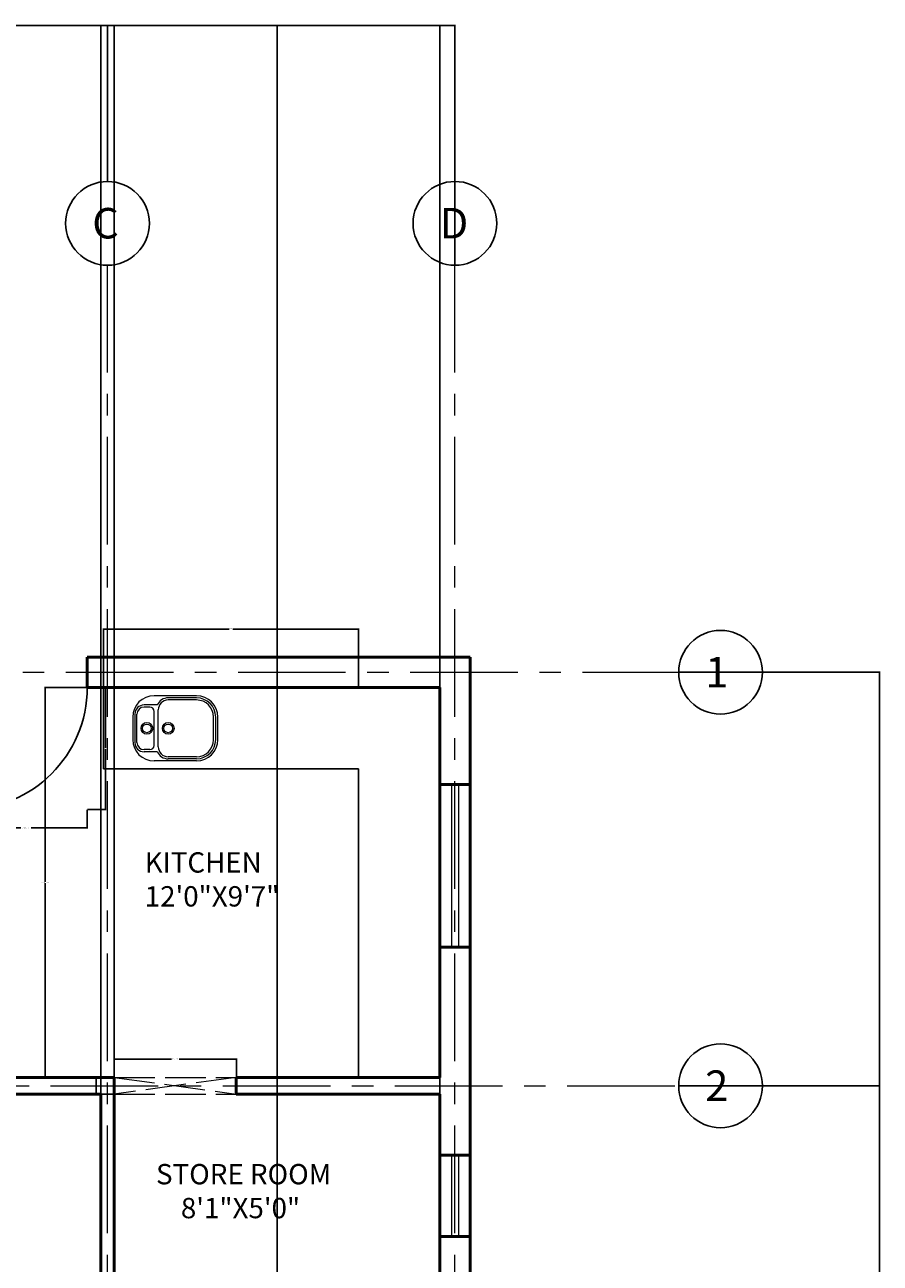
# Model space of a CAD drawing. Units: inches. Extents: x 10696 to 11614, y 5787 to 6498.
# Tile 9 of 9: x 11361 to 11614, y 6132 to 6498. Entities that reach past the tile are written whole.
import ezdxf

# ---------------------------------------------------------------- set-up
doc = ezdxf.new("R2010")
doc.units = ezdxf.units.IN
doc.linetypes.add('ACAD_ISO02W100', pattern=[15, 12, -3])
doc.linetypes.add('CENTER', pattern=[50.8, 31.75, -6.35, 6.35, -6.35])
for name, color, linetype, lineweight in [('A-ANNO-DIMS', 2, 'Continuous', 18), ('A-AREA-IDEN', 7, 'Continuous', 25), ('A-DOOR', 3, 'Continuous', 25), ('A-FLOR-CASE', 32, 'Continuous', 25), ('A-FLOR-FIXT', 9, 'Continuous', 20), ('A-GLAZ', 4, 'Continuous', 20), ('A-GRID', 1, 'CENTER', 18), ('A-GRID-IDEN', 1, 'Continuous', 25), ('A-WALL', 7, 'Continuous', 50), ('A-WALL-OVHD', 7, 'ACAD_ISO02W100', 18)]:
    doc.layers.add(name, color=color, linetype=linetype, lineweight=lineweight)
doc.styles.get("Standard").update_dxf_attribs({"font": 'arial.ttf'})
doc.dimstyles.get("Standard").update_dxf_attribs({"dimtxt": 0.18, "dimasz": 0.18, "dimexe": 0.18, "dimexo": 0.0625, "dimgap": 0.09, "dimtad": 0, "dimtih": 1, "dimtoh": 1, "dimdec": 4, "dimzin": 0, "dimdsep": 46, "dimtxsty": 'Standard', "dimcen": 0.09, "dimadec": 0, "dimazin": 0, "dimtfac": 1, "dimtdec": 4, "dimtofl": 0, "dimtmove": 0, "dimatfit": 3, "dimfxl": 1, "dimtolj": 1, "dimtzin": 0, "dimarcsym": 0})

# ---------------------------------------------------------------- blocks, each defined once
blk = doc.blocks.new('A$C29210457')
for p, q in [((0.63, 0.644), (0.21, 0.644)), ((0.63, 0.623), (0.35, 0.623)), ((0.242, 0.553), (0.112, 0.553)), ((0.168, 0.532), (0.112, 0.532)), ((0.14, 0.532), (0.14, 0.532)), ((0.21, 0.154), (0.21, 0.49)), ((0.252, 0.14), (0.252, 0.504)), ((0.63, 0.602), (0.35, 0.602)), ((0, 0.434), (0, 0.21)), ((0.021, 0.462), (0.021, 0.182)), ((0.042, 0.182), (0.042, 0.462)), ((0.798, 0.21), (0.798, 0.434)), ((0.819, 0.21), (0.819, 0.434)), ((0.84, 0.21), (0.84, 0.434)), ((0.168, 0.112), (0.112, 0.112)), ((0.242, 0.091), (0.112, 0.091)), ((0.14, 0.112), (0.14, 0.112)), ((0.63, 0), (0.21, 0)), ((0.63, 0.042), (0.35, 0.042)), ((0.63, 0.021), (0.35, 0.021))]:
    blk.add_line(p, q)
for centre, radius in [((0.14, 0.322), 0.0574), ((0.35, 0.322), 0.0574), ((0.14, 0.322), 0.0427), ((0.35, 0.322), 0.0427)]:
    blk.add_circle(centre, radius)
for centre, radius, start, end in [((0.21, 0.434), 0.21, 90, 180), ((0.35, 0.504), 0.119, 90.0649, 155.684), ((0.63, 0.434), 0.21, 0, 90), ((0.63, 0.434), 0.189, 0, 90), ((0.112, 0.462), 0.091, 90.0958, 180), ((0.112, 0.462), 0.07, 90, 180), ((0.168, 0.49), 0.042, 0, 90), ((0.35, 0.504), 0.098, 90, 180), ((0.63, 0.434), 0.168, 0, 90), ((0.21, 0.21), 0.21, 180, 270), ((0.112, 0.182), 0.091, 180, 270), ((0.112, 0.182), 0.07, 180, 270), ((0.168, 0.154), 0.042, 270, 0), ((0.35, 0.14), 0.098, 180, 270), ((0.63, 0.21), 0.21, 270, 0), ((0.63, 0.21), 0.168, 270, 0), ((0.63, 0.21), 0.189, 270, 0), ((0.35, 0.14), 0.119, 204.316, 269.978)]:
    blk.add_arc(centre, radius, start, end)
blk = doc.blocks.new('A$C292E2DA8')
at = {"xscale": 729, "yscale": 729, "zscale": 729}
blk.add_blockref('A$C29210457', (0, 0), dxfattribs=at)
blk = doc.blocks.new('DOOR-SINGLE-36-KITCHEN')
blk.add_line((0, 36), (0, 0))
blk.add_arc((0, 36), 36, 270, 0)
blk = doc.blocks.new('WIN-GLAZ-24')
for p, q in [((0, 24), (0, 0)), ((2, 24), (2, 0))]:
    blk.add_line(p, q)
blk = doc.blocks.new('WIN-GLAZ-48')
for p, q in [((0, 48), (0, 0)), ((2, 48), (2, 0))]:
    blk.add_line(p, q)
blk = doc.blocks.new('KITCHEN-COUNTER-L')
for p, q in [((0, 91), (0, 115)), ((0, 91), (75.19, 91)), ((75.19, 0), (75.19, 91))]:
    blk.add_line(p, q)
blk = doc.blocks.new('OPENING-OVHD-36X5')
for p, q in [((0, 5), (36, 5)), ((36, 5), (0, 0)), ((0, 5), (36, 0)), ((0, 0), (36, 0))]:
    blk.add_line(p, q)
blk = doc.blocks.new('*D48')
at = {"layer": 'A-ANNO-DIMS', "color": 0, "lineweight": -2, "transparency": 16777216}
for p, q in [((11343.77, 6266.01), (11343.77, 6260.49)), ((11379.77, 6266.01), (11379.77, 6260.49)), ((11343.95, 6260.67), (11360.24, 6260.67)), ((11379.59, 6260.67), (11363.29, 6260.67))]:
    blk.add_line(p, q, dxfattribs=at)
at = {"layer": 'A-ANNO-DIMS', "color": 0, "transparency": 16777216}
for points in [[(11343.95, 6260.7), (11343.95, 6260.64), (11343.77, 6260.67)], [(11379.59, 6260.7), (11379.59, 6260.64), (11379.77, 6260.67)]]:
    blk.add_solid(points, dxfattribs=at)
at = {"layer": 'Defpoints', "color": 0, "transparency": 16777216}
for p in [(11343.77, 6266.07), (11379.77, 6266.07), (11379.77, 6260.67)]:
    blk.add_point(p, dxfattribs=at)
at = {"layer": 'A-ANNO-DIMS', "color": 0, "transparency": 16777216, "insert": (11361.77, 6260.67), "char_height": 0.18, "attachment_point": 5}
blk.add_mtext('\\A1;KITCHEN DOOR 36 TYP.', dxfattribs=at)
blk = doc.blocks.new('*D49')
at = {"layer": 'A-ANNO-DIMS', "color": 0, "lineweight": -2, "transparency": 16777216}
for p, q in [((11379.83, 6302.07), (11385.35, 6302.07)), ((11385.17, 6301.89), (11385.17, 6284.25)), ((11385.17, 6266.25), (11385.17, 6283.89)), ((11379.83, 6266.07), (11385.35, 6266.07))]:
    blk.add_line(p, q, dxfattribs=at)
at = {"layer": 'A-ANNO-DIMS', "color": 0, "transparency": 16777216}
for points in [[(11385.14, 6301.89), (11385.2, 6301.89), (11385.17, 6302.07)], [(11385.14, 6266.25), (11385.2, 6266.25), (11385.17, 6266.07)]]:
    blk.add_solid(points, dxfattribs=at)
at = {"layer": 'Defpoints', "color": 0, "transparency": 16777216}
for p in [(11379.77, 6302.07), (11385.17, 6302.07), (11379.77, 6266.07)]:
    blk.add_point(p, dxfattribs=at)
at = {"layer": 'A-ANNO-DIMS', "color": 0, "transparency": 16777216, "insert": (11385.17, 6284.07), "char_height": 0.18, "attachment_point": 5}
blk.add_mtext('\\A1;36 TYP.', dxfattribs=at)
blk = doc.blocks.new('*D58')
at = {"layer": 'A-ANNO-DIMS', "color": 0, "lineweight": -2, "transparency": 16777216}
for p, q in [((11384.52, 6302.07), (11367.15, 6302.07)), ((11367.33, 6301.89), (11367.33, 6244.75)), ((11367.33, 6187.25), (11367.33, 6244.39)), ((11384.52, 6187.07), (11367.15, 6187.07))]:
    blk.add_line(p, q, dxfattribs=at)
at = {"layer": 'A-ANNO-DIMS', "color": 0, "transparency": 16777216}
for points in [[(11367.3, 6301.89), (11367.36, 6301.89), (11367.33, 6302.07)], [(11367.3, 6187.25), (11367.36, 6187.25), (11367.33, 6187.07)]]:
    blk.add_solid(points, dxfattribs=at)
at = {"layer": 'Defpoints', "color": 0, "transparency": 16777216}
for p in [(11367.33, 6302.07), (11384.58, 6302.07), (11384.58, 6187.07)]:
    blk.add_point(p, dxfattribs=at)
at = {"layer": 'A-ANNO-DIMS', "color": 0, "transparency": 16777216, "insert": (11367.33, 6244.57), "char_height": 0.18, "attachment_point": 5}
blk.add_mtext('\\A1;COUNTER 115 TYP.', dxfattribs=at)
blk = doc.blocks.new('*D59')
at = {"layer": 'A-ANNO-DIMS', "color": 0, "lineweight": -2, "transparency": 16777216}
for p, q in [((11384.58, 6302.13), (11384.58, 6319.5)), ((11384.76, 6319.32), (11421.65, 6319.32)), ((11459.59, 6319.32), (11422.7, 6319.32)), ((11459.77, 6302.13), (11459.77, 6319.5))]:
    blk.add_line(p, q, dxfattribs=at)
at = {"layer": 'A-ANNO-DIMS', "color": 0, "transparency": 16777216}
for points in [[(11384.76, 6319.35), (11384.76, 6319.29), (11384.58, 6319.32)], [(11459.59, 6319.35), (11459.59, 6319.29), (11459.77, 6319.32)]]:
    blk.add_solid(points, dxfattribs=at)
at = {"layer": 'Defpoints', "color": 0, "transparency": 16777216}
for p in [(11459.77, 6319.32), (11384.58, 6302.07), (11459.77, 6302.07)]:
    blk.add_point(p, dxfattribs=at)
at = {"layer": 'A-ANNO-DIMS', "color": 0, "transparency": 16777216, "insert": (11422.17, 6319.32), "char_height": 0.18, "attachment_point": 5}
blk.add_mtext('\\A1;75 TYP.', dxfattribs=at)
blk = doc.blocks.new('*D66')
at = {"layer": 'A-ANNO-DIMS', "color": 0, "lineweight": -2, "transparency": 16777216}
for p, q in [((11387.77, 6187.13), (11387.77, 6192.65)), ((11387.95, 6192.47), (11404.63, 6192.47)), ((11423.59, 6192.47), (11406.91, 6192.47)), ((11423.77, 6187.13), (11423.77, 6192.65))]:
    blk.add_line(p, q, dxfattribs=at)
at = {"layer": 'A-ANNO-DIMS', "color": 0, "transparency": 16777216}
for points in [[(11387.95, 6192.5), (11387.95, 6192.44), (11387.77, 6192.47)], [(11423.59, 6192.5), (11423.59, 6192.44), (11423.77, 6192.47)]]:
    blk.add_solid(points, dxfattribs=at)
at = {"layer": 'Defpoints', "color": 0, "transparency": 16777216}
for p in [(11423.77, 6192.47), (11387.77, 6187.07), (11423.77, 6187.07)]:
    blk.add_point(p, dxfattribs=at)
at = {"layer": 'A-ANNO-DIMS', "color": 0, "transparency": 16777216, "insert": (11405.77, 6192.47), "char_height": 0.18, "attachment_point": 5}
blk.add_mtext('\\A1;OPENING 36 TYP.', dxfattribs=at)
blk = doc.blocks.new('*D67')
at = {"layer": 'A-ANNO-DIMS', "color": 0, "lineweight": -2, "transparency": 16777216}
for p, q in [((11387.7, 6187.07), (11382.19, 6187.07)), ((11382.37, 6186.89), (11382.37, 6184.75)), ((11382.37, 6182.25), (11382.37, 6184.39)), ((11387.7, 6182.07), (11382.19, 6182.07))]:
    blk.add_line(p, q, dxfattribs=at)
at = {"layer": 'A-ANNO-DIMS', "color": 0, "transparency": 16777216}
for points in [[(11382.34, 6186.89), (11382.4, 6186.89), (11382.37, 6187.07)], [(11382.34, 6182.25), (11382.4, 6182.25), (11382.37, 6182.07)]]:
    blk.add_solid(points, dxfattribs=at)
at = {"layer": 'Defpoints', "color": 0, "transparency": 16777216}
for p in [(11382.37, 6187.07), (11387.77, 6187.07), (11387.77, 6182.07)]:
    blk.add_point(p, dxfattribs=at)
at = {"layer": 'A-ANNO-DIMS', "color": 0, "transparency": 16777216, "insert": (11382.37, 6184.57), "char_height": 0.18, "attachment_point": 5}
blk.add_mtext('\\A1;5 TYP.', dxfattribs=at)
blk = doc.blocks.new('*D78')
at = {"layer": 'A-ANNO-DIMS', "color": 0, "lineweight": -2, "transparency": 16777216}
for p, q in [((11335.27, 6451.45), (11335.27, 6497.62)), ((11335.45, 6497.44), (11360.19, 6497.44)), ((11385.59, 6497.44), (11360.84, 6497.44)), ((11385.77, 6451.45), (11385.77, 6497.62))]:
    blk.add_line(p, q, dxfattribs=at)
at = {"layer": 'A-ANNO-DIMS', "color": 0, "transparency": 16777216}
for points in [[(11335.45, 6497.47), (11335.45, 6497.41), (11335.27, 6497.44)], [(11385.59, 6497.47), (11385.59, 6497.41), (11385.77, 6497.44)]]:
    blk.add_solid(points, dxfattribs=at)
at = {"layer": 'Defpoints', "color": 0, "transparency": 16777216}
for p in [(11385.77, 6497.44), (11335.27, 6451.39), (11385.77, 6451.39)]:
    blk.add_point(p, dxfattribs=at)
at = {"layer": 'A-ANNO-DIMS', "color": 0, "transparency": 16777216, "insert": (11360.52, 6497.44), "char_height": 0.18, "attachment_point": 5}
blk.add_mtext('\\A1;50.5', dxfattribs=at)
blk = doc.blocks.new('*D79')
at = {"layer": 'A-ANNO-DIMS', "color": 0, "lineweight": -2, "transparency": 16777216}
for p, q in [((11385.77, 6451.45), (11385.77, 6497.62)), ((11385.95, 6497.44), (11436.63, 6497.44)), ((11488.09, 6497.44), (11437.4, 6497.44)), ((11488.27, 6451.45), (11488.27, 6497.62))]:
    blk.add_line(p, q, dxfattribs=at)
at = {"layer": 'A-ANNO-DIMS', "color": 0, "transparency": 16777216}
for points in [[(11385.95, 6497.47), (11385.95, 6497.41), (11385.77, 6497.44)], [(11488.09, 6497.47), (11488.09, 6497.41), (11488.27, 6497.44)]]:
    blk.add_solid(points, dxfattribs=at)
at = {"layer": 'Defpoints', "color": 0, "transparency": 16777216}
for p in [(11488.27, 6497.44), (11385.77, 6451.39), (11488.27, 6451.39)]:
    blk.add_point(p, dxfattribs=at)
at = {"layer": 'A-ANNO-DIMS', "color": 0, "transparency": 16777216, "insert": (11437.02, 6497.44), "char_height": 0.18, "attachment_point": 5}
blk.add_mtext('\\A1;102.5', dxfattribs=at)
blk = doc.blocks.new('*D80')
at = {"layer": 'A-ANNO-DIMS', "color": 0, "lineweight": -2, "transparency": 16777216}
for p, q in [((11170.27, 6426.74), (11170.27, 6497.62)), ((11170.45, 6497.44), (11328.98, 6497.44)), ((11488.09, 6497.44), (11329.56, 6497.44)), ((11488.27, 6426.74), (11488.27, 6497.62))]:
    blk.add_line(p, q, dxfattribs=at)
at = {"layer": 'A-ANNO-DIMS', "color": 0, "transparency": 16777216}
for points in [[(11170.45, 6497.47), (11170.45, 6497.41), (11170.27, 6497.44)], [(11488.09, 6497.47), (11488.09, 6497.41), (11488.27, 6497.44)]]:
    blk.add_solid(points, dxfattribs=at)
at = {"layer": 'Defpoints', "color": 0, "transparency": 16777216}
for p in [(11488.27, 6497.44), (11170.27, 6426.68), (11488.27, 6426.68)]:
    blk.add_point(p, dxfattribs=at)
at = {"layer": 'A-ANNO-DIMS', "color": 0, "transparency": 16777216, "insert": (11329.27, 6497.44), "char_height": 0.18, "attachment_point": 5}
blk.add_mtext('\\A1;318', dxfattribs=at)
blk = doc.blocks.new('*D81')
at = {"layer": 'A-ANNO-DIMS', "color": 0, "lineweight": -2, "transparency": 16777216}
for p, q in [((11554.32, 6306.57), (11613.7, 6306.57)), ((11613.52, 6306.39), (11613.52, 6245.75)), ((11613.52, 6184.75), (11613.52, 6245.39)), ((11554.32, 6184.57), (11613.7, 6184.57))]:
    blk.add_line(p, q, dxfattribs=at)
at = {"layer": 'A-ANNO-DIMS', "color": 0, "transparency": 16777216}
for points in [[(11613.49, 6306.39), (11613.55, 6306.39), (11613.52, 6306.57)], [(11613.49, 6184.75), (11613.55, 6184.75), (11613.52, 6184.57)]]:
    blk.add_solid(points, dxfattribs=at)
at = {"layer": 'Defpoints', "color": 0, "transparency": 16777216}
for p in [(11554.26, 6306.57), (11554.26, 6184.57), (11613.52, 6184.57)]:
    blk.add_point(p, dxfattribs=at)
at = {"layer": 'A-ANNO-DIMS', "color": 0, "transparency": 16777216, "insert": (11613.52, 6245.57), "char_height": 0.18, "attachment_point": 5}
blk.add_mtext('\\A1;122', dxfattribs=at)
blk = doc.blocks.new('*D82')
at = {"layer": 'A-ANNO-DIMS', "color": 0, "lineweight": -2, "transparency": 16777216}
for p, q in [((11554.32, 6184.57), (11613.7, 6184.57)), ((11613.52, 6184.39), (11613.52, 6152.25)), ((11613.52, 6119.75), (11613.52, 6151.89)), ((11554.32, 6119.57), (11613.7, 6119.57))]:
    blk.add_line(p, q, dxfattribs=at)
at = {"layer": 'A-ANNO-DIMS', "color": 0, "transparency": 16777216}
for points in [[(11613.49, 6184.39), (11613.55, 6184.39), (11613.52, 6184.57)], [(11613.49, 6119.75), (11613.55, 6119.75), (11613.52, 6119.57)]]:
    blk.add_solid(points, dxfattribs=at)
at = {"layer": 'Defpoints', "color": 0, "transparency": 16777216}
for p in [(11554.26, 6184.57), (11554.26, 6119.57), (11613.52, 6119.57)]:
    blk.add_point(p, dxfattribs=at)
at = {"layer": 'A-ANNO-DIMS', "color": 0, "transparency": 16777216, "insert": (11613.52, 6152.07), "char_height": 0.18, "attachment_point": 5}
blk.add_mtext('\\A1;65', dxfattribs=at)
blk = doc.blocks.new('*D86')
at = {"layer": 'A-ANNO-DIMS', "color": 0, "lineweight": -2, "transparency": 16777216}
for p, q in [((11579.03, 6306.57), (11613.7, 6306.57)), ((11613.52, 6306.39), (11613.52, 6131.75)), ((11613.52, 5956.75), (11613.52, 6131.39)), ((11579.03, 5956.57), (11613.7, 5956.57))]:
    blk.add_line(p, q, dxfattribs=at)
at = {"layer": 'A-ANNO-DIMS', "color": 0, "transparency": 16777216}
for points in [[(11613.49, 6306.39), (11613.55, 6306.39), (11613.52, 6306.57)], [(11613.49, 5956.75), (11613.55, 5956.75), (11613.52, 5956.57)]]:
    blk.add_solid(points, dxfattribs=at)
at = {"layer": 'Defpoints', "color": 0, "transparency": 16777216}
for p in [(11578.97, 6306.57), (11578.97, 5956.57), (11613.52, 5956.57)]:
    blk.add_point(p, dxfattribs=at)
at = {"layer": 'A-ANNO-DIMS', "color": 0, "transparency": 16777216, "insert": (11613.52, 6131.57), "char_height": 0.18, "attachment_point": 5}
blk.add_mtext('\\A1;350', dxfattribs=at)
blk = doc.blocks.new('*D94')
at = {"layer": 'A-ANNO-DIMS', "color": 0, "lineweight": -2, "transparency": 16777216}
for p, q in [((11435.77, 5896.13), (11435.77, 6497.62)), ((11435.95, 6497.44), (11459.54, 6497.44)), ((11483.59, 6497.44), (11459.99, 6497.44)), ((11483.77, 5896.13), (11483.77, 6497.62))]:
    blk.add_line(p, q, dxfattribs=at)
at = {"layer": 'A-ANNO-DIMS', "color": 0, "transparency": 16777216}
for points in [[(11435.95, 6497.47), (11435.95, 6497.41), (11435.77, 6497.44)], [(11483.59, 6497.47), (11483.59, 6497.41), (11483.77, 6497.44)]]:
    blk.add_solid(points, dxfattribs=at)
at = {"layer": 'Defpoints', "color": 0, "transparency": 16777216}
for p in [(11435.77, 6497.44), (11435.77, 5896.07), (11483.77, 5896.07)]:
    blk.add_point(p, dxfattribs=at)
at = {"layer": 'A-ANNO-DIMS', "color": 0, "transparency": 16777216, "insert": (11459.77, 6497.44), "char_height": 0.18, "attachment_point": 5}
blk.add_mtext('\\A1;48', dxfattribs=at)
blk = doc.blocks.new('*D99')
at = {"layer": 'A-ANNO-DIMS', "color": 0, "lineweight": -2, "transparency": 16777216}
for p, q in [((11383.77, 6182.13), (11383.77, 6497.62)), ((11383.95, 6497.44), (11385.62, 6497.44)), ((11387.59, 6497.44), (11385.92, 6497.44)), ((11387.77, 6182.13), (11387.77, 6497.62))]:
    blk.add_line(p, q, dxfattribs=at)
at = {"layer": 'A-ANNO-DIMS', "color": 0, "transparency": 16777216}
for points in [[(11383.95, 6497.47), (11383.95, 6497.41), (11383.77, 6497.44)], [(11387.59, 6497.47), (11387.59, 6497.41), (11387.77, 6497.44)]]:
    blk.add_solid(points, dxfattribs=at)
at = {"layer": 'Defpoints', "color": 0, "transparency": 16777216}
for p in [(11387.77, 6497.44), (11383.77, 6182.07), (11387.77, 6182.07)]:
    blk.add_point(p, dxfattribs=at)
at = {"layer": 'A-ANNO-DIMS', "color": 0, "transparency": 16777216, "insert": (11385.77, 6497.44), "char_height": 0.18, "attachment_point": 5}
blk.add_mtext('\\A1;4', dxfattribs=at)

msp = doc.modelspace()

# ---------------------------------------------------------------- linework, layer by layer
at = {"layer": 'A-GRID'}
for p, q in [((11385.767, 5887.07), (11385.767, 6426.679)), ((11488.267, 5887.07), (11488.267, 6426.679)), ((11170.267, 6306.57), (11554.26, 6306.57)), ((11165.767, 6184.57), (11554.26, 6184.57))]:
    msp.add_line(p, q, dxfattribs=at)
at = {"layer": 'A-GRID-IDEN'}
for centre in [(11385.767, 6439.033), (11488.267, 6439.033), (11566.613, 6306.57), (11566.613, 6184.57)]:
    msp.add_circle(centre, 12.353, dxfattribs=at)
at = {"layer": 'A-WALL'}
for p, q in [((11379.767, 6311.07), (11492.767, 6311.07)), ((11379.767, 6302.07), (11379.767, 6311.07)), ((11492.767, 5887.07), (11492.767, 6311.07)), ((11379.767, 6302.07), (11483.767, 6302.07)), ((11483.767, 6187.07), (11483.767, 6302.07)), ((11483.767, 6273.514), (11492.767, 6273.514)), ((11483.767, 6225.514), (11492.767, 6225.514)), ((11330.767, 6187.07), (11387.767, 6187.07)), ((11387.767, 6122.07), (11387.767, 6187.07)), ((11423.767, 6187.07), (11483.767, 6187.07)), ((11423.767, 6182.07), (11423.767, 6187.07)), ((11330.767, 6182.07), (11383.767, 6182.07)), ((11383.767, 6113.07), (11383.767, 6182.07)), ((11423.767, 6182.07), (11483.767, 6182.07)), ((11483.767, 6122.07), (11483.767, 6182.07)), ((11483.767, 6164.07), (11492.767, 6164.07)), ((11483.767, 6140.07), (11492.767, 6140.07))]:
    msp.add_line(p, q, dxfattribs=at)

# ---------------------------------------------------------------- block references
at = {"layer": 'A-DOOR'}
msp.add_blockref('DOOR-SINGLE-36-KITCHEN', (11343.767, 6266.07), dxfattribs=at)
at = {"layer": 'A-FLOR-CASE'}
msp.add_blockref('KITCHEN-COUNTER-L', (11384.578, 6187.07), dxfattribs=at)
at = {"layer": 'A-FLOR-FIXT', "xscale": 0.0409818961513061, "yscale": 0.0409818961513061, "zscale": 0.0409818961513061}
msp.add_blockref('A$C292E2DA8', (11393.208, 6280.417), dxfattribs=at)
at = {"layer": 'A-GLAZ'}
for name, p in [('WIN-GLAZ-48', (11487.267, 6225.514)), ('WIN-GLAZ-24', (11487.267, 6140.07))]:
    msp.add_blockref(name, p, dxfattribs=at)
at = {"layer": 'A-WALL-OVHD'}
msp.add_blockref('OPENING-OVHD-36X5', (11387.767, 6182.07), dxfattribs=at)

# ---------------------------------------------------------------- texts
at = {"layer": 'A-AREA-IDEN', "char_height": 6, "attachment_point": 1}
for s, width, insert in [('KITCHEN\\P12\'0"X9\'7"', 38.38274, (11396.738, 6253.474)), ('STORE ROOM\\P    8\'1"X5\'0"', 59.23595, (11400.075, 6161.5))]:
    msp.add_mtext_dynamic_manual_height_columns(s, width=width, gutter_width=12.5, heights=[0], dxfattribs=dict(at, insert=insert))
at = {"layer": 'A-GRID-IDEN', "char_height": 9, "attachment_point": 1}
for s, insert in [('C', (11381.257, 6443.573)), ('D', (11483.757, 6443.573)), ('1', (11562.102, 6311.11)), ('2', (11562.102, 6189.11))]:
    msp.add_mtext_dynamic_manual_height_columns(s, width=18.12678, gutter_width=12.5, heights=[0], dxfattribs=dict(at, insert=insert))

# ---------------------------------------------------------------- dimensions: what is measured, and where the dimension line sits
at = {"layer": 'A-ANNO-DIMS'}
for base, p1, p2, override, picture, middle in [((11488.267, 6497.443), (11170.267, 6426.679), (11488.267, 6426.679), {"dimdec": 0, "dimlfac": 1, "dimrnd": 0, "dimzin": 0, "dimdsep": 46, "dimlunit": 2}, '*D80', (11329.267, 6497.443)), ((11385.767, 6497.443), (11335.267, 6451.386), (11385.767, 6451.386), {"dimdec": 1, "dimlfac": 1, "dimrnd": 0, "dimzin": 0, "dimdsep": 46, "dimlunit": 2}, '*D78', (11360.517, 6497.443)), ((11387.767, 6497.443), (11383.767, 6182.07), (11387.767, 6182.07), {"dimdec": 0, "dimlfac": 1, "dimrnd": 0, "dimzin": 0, "dimdsep": 46, "dimlunit": 2}, '*D99', (11385.767, 6497.443)), ((11488.267, 6497.443), (11385.767, 6451.386), (11488.267, 6451.386), {"dimdec": 1, "dimlfac": 1, "dimrnd": 0, "dimzin": 0, "dimdsep": 46, "dimlunit": 2}, '*D79', (11437.017, 6497.443)), ((11435.767, 6497.443), (11483.767, 5896.07), (11435.767, 5896.07), {"dimdec": 0, "dimlfac": 1, "dimrnd": 0, "dimzin": 0, "dimdsep": 46, "dimlunit": 2}, '*D94', (11459.767, 6497.443))]:
    dim = msp.add_linear_dim(base=base, p1=p1, p2=p2, dimstyle='Standard', override=override, dxfattribs=at)
    dim.commit()
    dim.dimension.update_dxf_attribs({"geometry": picture, "text_midpoint": middle})
for base, p1, p2, text, picture, middle in [((11459.767, 6319.32), (11384.578, 6302.07), (11459.767, 6302.07), '<> TYP.', '*D59', (11422.173, 6319.32)), ((11379.767, 6260.67), (11343.767, 6266.07), (11379.767, 6266.07), 'KITCHEN DOOR <> TYP.', '*D48', (11361.767, 6260.67)), ((11423.767, 6192.47), (11387.767, 6187.07), (11423.767, 6187.07), 'OPENING <> TYP.', '*D66', (11405.767, 6192.47))]:
    dim = msp.add_linear_dim(base=base, p1=p1, p2=p2, text=text, dimstyle='Standard', override={"dimdec": 0, "dimlfac": 1, "dimrnd": 0, "dimzin": 0, "dimdsep": 46, "dimlunit": 2}, dxfattribs=at)
    dim.commit()
    dim.dimension.update_dxf_attribs({"geometry": picture, "text_midpoint": middle})
for base, p1, p2, picture, middle in [((11613.516, 6184.57), (11554.26, 6306.57), (11554.26, 6184.57), '*D81', (11613.516, 6245.57)), ((11613.516, 5956.57), (11578.966, 6306.57), (11578.966, 5956.57), '*D86', (11613.516, 6131.57)), ((11613.516, 6119.57), (11554.26, 6184.57), (11554.26, 6119.57), '*D82', (11613.516, 6152.07))]:
    dim = msp.add_linear_dim(base=base, p1=p1, p2=p2, angle=90, dimstyle='Standard', override={"dimdec": 0, "dimlfac": 1, "dimrnd": 0, "dimzin": 0, "dimdsep": 46, "dimlunit": 2}, dxfattribs=at)
    dim.commit()
    dim.dimension.update_dxf_attribs({"geometry": picture, "text_midpoint": middle})
for base, p1, p2, text, picture, middle in [((11367.328, 6302.07), (11384.578, 6187.07), (11384.578, 6302.07), 'COUNTER <> TYP.', '*D58', (11367.328, 6244.57)), ((11385.167, 6302.07), (11379.767, 6266.07), (11379.767, 6302.07), '<> TYP.', '*D49', (11385.167, 6284.07)), ((11382.367, 6187.07), (11387.767, 6182.07), (11387.767, 6187.07), '<> TYP.', '*D67', (11382.367, 6184.57))]:
    dim = msp.add_linear_dim(base=base, p1=p1, p2=p2, angle=90, text=text, dimstyle='Standard', override={"dimdec": 0, "dimlfac": 1, "dimrnd": 0, "dimzin": 0, "dimdsep": 46, "dimlunit": 2}, dxfattribs=at)
    dim.commit()
    dim.dimension.update_dxf_attribs({"geometry": picture, "text_midpoint": middle})

doc.saveas('drawing.dxf')
